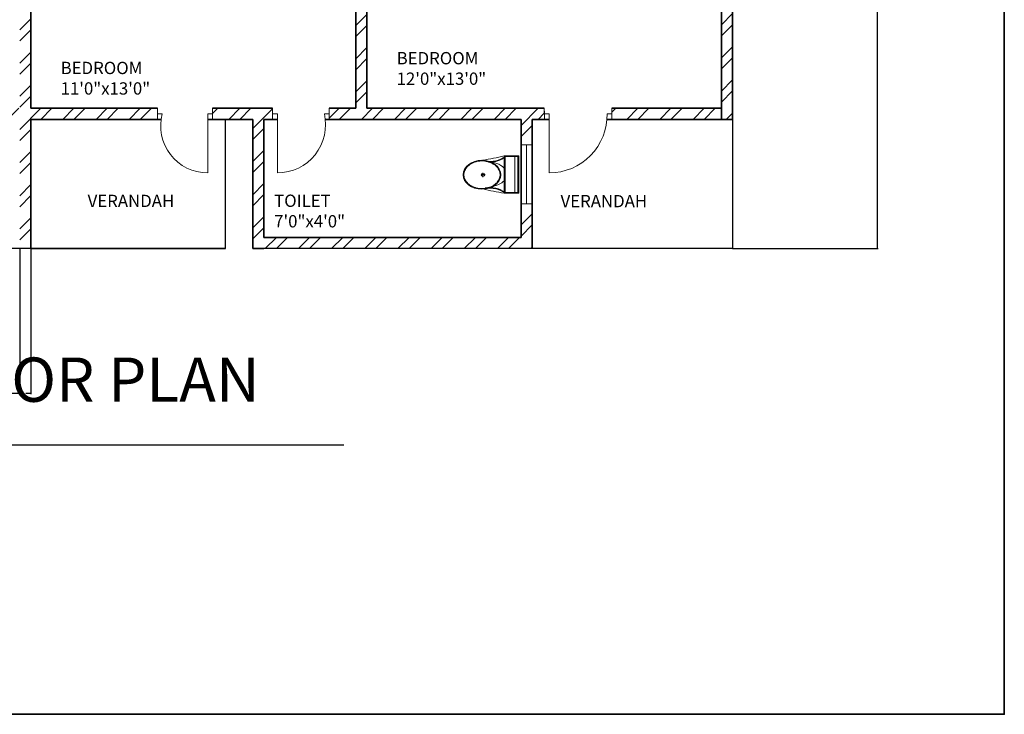
# Model space of a CAD drawing. Units: inches. Extents: x 1962 to 2771, y 1245 to 2660.
# Tile 8 of 114: x 2371 to 2771, y 1245 to 1527. Entities that reach past the tile are written whole.
import ezdxf

# ---------------------------------------------------------------- set-up
doc = ezdxf.new("R2010")
doc.units = ezdxf.units.IN
for name, color, linetype, lineweight in [('A-ANNO-DIMS', 2, 'Continuous', 18), ('A-ANNO-TEXT', 7, 'Continuous', 25), ('A-ANNO-TTLB', 7, 'Continuous', 35), ('A-AREA-IDEN', 7, 'Continuous', 18), ('A-DOOR', 3, 'Continuous', 18), ('A-FLOR-BALC', 7, 'Continuous', 25), ('A-FLOR-FIXT', 8, 'Continuous', 18), ('A-GLAZ', 4, 'Continuous', 18), ('A-WALL', 7, 'Continuous', 35), ('A-WALL-PATT', 252, 'Continuous', 13)]:
    doc.layers.add(name, color=color, linetype=linetype, lineweight=lineweight)
doc.styles.get("Standard").update_dxf_attribs({"font": 'arial.ttf'})
doc.dimstyles.get("Standard").update_dxf_attribs({"dimtxt": 0.18, "dimasz": 0.18, "dimexe": 0.18, "dimexo": 0.0625, "dimgap": 0.09, "dimtad": 0, "dimtih": 1, "dimtoh": 1, "dimdec": 4, "dimzin": 0, "dimdsep": 46, "dimtxsty": 'Standard', "dimcen": 0.09, "dimadec": 0, "dimazin": 0, "dimtfac": 1, "dimtdec": 4, "dimtofl": 0, "dimtmove": 0, "dimatfit": 3, "dimfxl": 1, "dimtolj": 1, "dimtzin": 0, "dimarcsym": 0})

# ---------------------------------------------------------------- blocks, each defined once
blk = doc.blocks.new('A$C31115884')
for p, q in [((283, 498), (223, 498)), ((258, 466), (258, 523)), ((0, 200), (0, 0)), ((520, 200), (0, 200)), ((10, 190), (10, 10)), ((510, 190), (10, 190)), ((510, 10), (510, 190)), ((520, 0), (520, 200)), ((510, 54), (0, 54)), ((10, 10), (510, 10)), ((0, 0), (520, 0))]:
    blk.add_line(p, q)
blk.add_circle((256, 496), 23.6)
for centre, radius, start, end in [((2778, -205), 2807, 165.4549, 171.7133), ((-295, 403), 365, 324.2091, 9.3499), ((-295, 403), 375, 324.2091, 9.3499), ((139, 406), 293, 315.8436, 2.6563), ((806, 403), 365, 170.6501, 215.7909), ((3237, 905), 2807, 188.2867, 194.5451), ((384, 406), 293, 190.2774, 224.1564), ((806, 403), 375, 179.2036, 215.7909)]:
    blk.add_arc(centre, radius, start, end)
blk.add_ellipse((256, 510), major_axis=(0, -261), ratio=0.772727)
blk.add_open_spline([(256, 259), (263, 259), (270, 260), (288, 262), (299, 265), (320, 273), (330, 278), (350, 291), (360, 299), (378, 316), (386, 326), (402, 347), (409, 358), (421, 383), (427, 395), (436, 422), (440, 436), (445, 465), (447, 480), (448, 509), (448, 524), (445, 553), (443, 568), (436, 596), (432, 610), (422, 636), (416, 649), (402, 672), (395, 683), (379, 703), (370, 712), (351, 728), (341, 735), (321, 746), (310, 751), (289, 757), (278, 759), (256, 761), (245, 761), (223, 757), (212, 754), (191, 746), (181, 741), (161, 728), (151, 720), (133, 703), (125, 693), (110, 672), (103, 660), (90, 636), (85, 623), (76, 596), (72, 582), (67, 553), (66, 538), (64, 509), (65, 494), (68, 465), (70, 450), (77, 422), (81, 408), (91, 382), (97, 370), (111, 346), (118, 335), (135, 316), (144, 307), (162, 291), (172, 284), (193, 273), (203, 269), (225, 262), (236, 260), (250, 259), (253, 259), (256, 259)], degree=3, knots=[0, 0, 0, 0, 0.110105, 0.110105, 0.285049, 0.285049, 0.459994, 0.459994, 0.634938, 0.634938, 0.809882, 0.809882, 0.984827, 0.984827, 1.159771, 1.159771, 1.334715, 1.334715, 1.50966, 1.50966, 1.684604, 1.684604, 1.859549, 1.859549, 2.034493, 2.034493, 2.209437, 2.209437, 2.384382, 2.384382, 2.559326, 2.559326, 2.73427, 2.73427, 2.909215, 2.909215, 3.084159, 3.084159, 3.259103, 3.259103, 3.434048, 3.434048, 3.608992, 3.608992, 3.783936, 3.783936, 3.958881, 3.958881, 4.133825, 4.133825, 4.30877, 4.30877, 4.483714, 4.483714, 4.658658, 4.658658, 4.833603, 4.833603, 5.008547, 5.008547, 5.183491, 5.183491, 5.358436, 5.358436, 5.53338, 5.53338, 5.708324, 5.708324, 5.883269, 5.883269, 6.058213, 6.058213, 6.233158, 6.233158, 6.283185, 6.283185, 6.283185, 6.283185])
blk = doc.blocks.new('WIN-24IN-A')
for p, q in [((0, 24), (4.5, 24)), ((4.5, 24), (2.25, 24)), ((2.25, 24), (2.25, 0)), ((2.25, 0), (0, 0)), ((0, 0), (4.5, 0))]:
    blk.add_line(p, q)
blk = doc.blocks.new('*D42')
at = {"layer": 'A-ANNO-DIMS', "color": 0, "lineweight": -2, "transparency": 16777216}
for p, q in [((2660.87, 2524.34), (2719.94, 2524.34)), ((2719.76, 2524.16), (2719.76, 1979.28)), ((2719.76, 1434.02), (2719.76, 1978.91)), ((2660.87, 1433.84), (2719.94, 1433.84))]:
    blk.add_line(p, q, dxfattribs=at)
at = {"layer": 'A-ANNO-DIMS', "color": 0, "transparency": 16777216}
for points in [[(2719.73, 2524.16), (2719.79, 2524.16), (2719.76, 2524.34)], [(2719.73, 1434.02), (2719.79, 1434.02), (2719.76, 1433.84)]]:
    blk.add_solid(points, dxfattribs=at)
at = {"layer": 'Defpoints', "color": 0, "transparency": 16777216}
for p in [(2660.81, 2524.34), (2719.76, 2524.34), (2660.81, 1433.84)]:
    blk.add_point(p, dxfattribs=at)
at = {"layer": 'A-ANNO-DIMS', "color": 0, "transparency": 16777216, "insert": (2719.76, 1979.09), "char_height": 0.18, "attachment_point": 5}
blk.add_mtext('\\A1;1090.5', dxfattribs=at)
blk = doc.blocks.new('*D46')
at = {"layer": 'A-ANNO-DIMS', "color": 0, "lineweight": -2, "transparency": 16777216}
for p, q in [((2086.31, 1433.78), (2086.31, 1374.71)), ((2371.31, 1433.78), (2371.31, 1374.71)), ((2086.49, 1374.89), (2228.52, 1374.89)), ((2371.13, 1374.89), (2229.1, 1374.89))]:
    blk.add_line(p, q, dxfattribs=at)
at = {"layer": 'A-ANNO-DIMS', "color": 0, "transparency": 16777216}
for points in [[(2086.49, 1374.92), (2086.49, 1374.86), (2086.31, 1374.89)], [(2371.13, 1374.92), (2371.13, 1374.86), (2371.31, 1374.89)]]:
    blk.add_solid(points, dxfattribs=at)
at = {"layer": 'Defpoints', "color": 0, "transparency": 16777216}
for p in [(2086.31, 1433.84), (2371.31, 1433.84), (2086.31, 1374.89)]:
    blk.add_point(p, dxfattribs=at)
at = {"layer": 'A-ANNO-DIMS', "color": 0, "transparency": 16777216, "insert": (2228.81, 1374.89), "char_height": 0.18, "attachment_point": 5}
blk.add_mtext('\\A1;285', dxfattribs=at)
blk = doc.blocks.new('*D48')
at = {"layer": 'A-ANNO-DIMS', "color": 0, "lineweight": -2, "transparency": 16777216}
for p, q in [((2371.31, 1433.78), (2371.31, 1374.71)), ((2375.81, 1433.78), (2375.81, 1374.71)), ((2371.49, 1374.89), (2373.3, 1374.89)), ((2375.63, 1374.89), (2373.82, 1374.89))]:
    blk.add_line(p, q, dxfattribs=at)
at = {"layer": 'A-ANNO-DIMS', "color": 0, "transparency": 16777216}
for points in [[(2371.49, 1374.92), (2371.49, 1374.86), (2371.31, 1374.89)], [(2375.63, 1374.92), (2375.63, 1374.86), (2375.81, 1374.89)]]:
    blk.add_solid(points, dxfattribs=at)
at = {"layer": 'Defpoints', "color": 0, "transparency": 16777216}
for p in [(2371.31, 1433.84), (2375.81, 1433.84), (2371.31, 1374.89)]:
    blk.add_point(p, dxfattribs=at)
at = {"layer": 'A-ANNO-DIMS', "color": 0, "transparency": 16777216, "insert": (2373.56, 1374.89), "char_height": 0.18, "attachment_point": 5}
blk.add_mtext('\\A1;4.5', dxfattribs=at)

msp = doc.modelspace()

# ---------------------------------------------------------------- hatches: boundary and pattern name
at = {"layer": 'A-WALL-PATT'}
h = msp.add_hatch(dxfattribs=at)
h.set_pattern_fill('ANSI32', color=256)
h.paths.add_polyline_path([(2090.8074, 2467.3437), (2141.6481, 2467.3437), (2141.6481, 2469.5937), (2141.6481, 2471.8437), (2086.3074, 2471.8437), (2086.3074, 2422.5333), (2090.8074, 2422.5333)])
h.paths.add_polyline_path([(2282.7664, 2471.8437), (2204.8982, 2471.8437), (2204.8982, 2467.3437), (2234.8074, 2467.3437), (2234.8074, 2311.3437), (2228.7492, 2311.3437), (2228.7492, 2306.8437), (2234.8074, 2306.8437), (2331.9227, 2306.8437), (2331.9227, 2309.0937), (2331.9227, 2311.3437), (2239.3074, 2311.3437), (2239.3074, 2467.3437), (2282.7664, 2467.3437), (2282.7664, 2469.5937)])
h.paths.add_polyline_path([(2471.4531, 2519.8437), (2552.011, 2519.8437), (2564.3996, 2519.8437), (2564.3996, 2511.1389), (2568.8996, 2511.1389), (2568.8996, 2524.3437), (2466.9531, 2524.3437), (2466.9531, 2471.8437), (2450.0749, 2471.8437), (2446.4672, 2471.8437), (2446.4672, 2467.3437), (2450.0749, 2467.3437), (2475.9988, 2467.3437), (2475.9988, 2469.5937), (2475.9988, 2471.8437), (2471.4531, 2471.8437)])
h.paths.add_polyline_path([(2575.2231, 2469.5937), (2575.2231, 2471.8437), (2568.8996, 2471.8437), (2568.8996, 2487.1389), (2564.3996, 2487.1389), (2564.3996, 2471.8437), (2556.511, 2471.8437), (2499.2904, 2471.8437), (2499.2904, 2467.3437), (2507.8074, 2467.3437), (2507.8074, 2311.3437), (2414.863, 2311.3437), (2414.863, 2306.8437), (2512.3074, 2306.8437), (2517.0114, 2306.8437), (2517.0114, 2309.0937), (2517.0114, 2311.3437), (2512.3074, 2311.3437), (2512.3074, 2467.3437), (2575.2231, 2467.3437)])
h.paths.add_polyline_path([(2660.8074, 2471.8437), (2600.9602, 2471.8437), (2600.9602, 2467.3437), (2656.3074, 2467.3437), (2656.3074, 2432.5704), (2660.8074, 2432.5704)])
h.paths.add_polyline_path([(2660.8074, 2372.5704), (2656.3074, 2372.5704), (2656.3074, 2311.3437), (2600.276, 2311.3437), (2600.276, 2309.0937), (2600.276, 2306.8437), (2656.3074, 2306.8437), (2656.3074, 2296.2593), (2660.8074, 2296.2593)])
h.paths.add_polyline_path([(2572.3074, 2306.8437), (2577.1385, 2306.8437), (2577.1385, 2311.3437), (2551.082, 2311.3437), (2551.082, 2306.8437), (2567.8074, 2306.8437), (2567.8074, 2258.8437), (2540.0574, 2258.8437), (2540.0574, 2256.5937), (2540.0574, 2254.3437), (2567.8074, 2254.3437), (2656.3074, 2254.3437), (2656.3074, 2236.9085), (2660.8074, 2236.9085), (2660.8074, 2272.2593), (2656.3074, 2272.2593), (2656.3074, 2258.8437), (2572.3074, 2258.8437)])
h.paths.add_polyline_path([(2512.3074, 2254.3437), (2518.8716, 2254.3437), (2518.8716, 2256.5937), (2518.8716, 2258.8437), (2507.8074, 2258.8437), (2507.8074, 2177.8437), (2567.8074, 2177.8437), (2567.8074, 2172.9628), (2572.3074, 2172.9628), (2572.3074, 2177.8437), (2656.3074, 2177.8437), (2656.3074, 2166.4846), (2660.8074, 2166.4846), (2660.8074, 2200.9085), (2656.3074, 2200.9085), (2656.3074, 2182.3437), (2512.3074, 2182.3437)])
h.paths.add_polyline_path([(2656.3074, 2129.8437), (2572.3074, 2129.8437), (2572.3074, 2150.3044), (2570.0574, 2150.3044), (2567.8074, 2150.3044), (2567.8074, 2129.8437), (2507.8074, 2129.8437), (2507.8074, 2116.3027), (2510.0574, 2116.3027), (2512.3074, 2116.3027), (2512.3074, 2125.3437), (2567.8074, 2125.3437), (2572.3074, 2125.3437), (2656.3074, 2125.3437)])
h.paths.add_polyline_path([(2090.8074, 2362.5333), (2086.3074, 2362.5333), (2086.3074, 2298.6242), (2090.8074, 2298.6242), (2090.8074, 2306.8437), (2174.8074, 2306.8437), (2174.8074, 2286.4178), (2179.3074, 2286.4178), (2179.3074, 2306.8437), (2192.8641, 2306.8437), (2192.8641, 2309.0937), (2192.8641, 2311.3437), (2090.8074, 2311.3437)])
h.paths.add_polyline_path([(2209.156, 2258.8437), (2179.3074, 2258.8437), (2179.3074, 2263.2236), (2177.0574, 2263.2236), (2174.8074, 2263.2236), (2174.8074, 2258.8437), (2090.8074, 2258.8437), (2090.8074, 2274.6242), (2086.3074, 2274.6242), (2086.3074, 2238.2967), (2088.5574, 2238.2967), (2090.8074, 2238.2967), (2090.8074, 2254.3437), (2209.156, 2254.3437)])
h.paths.add_polyline_path([(2090.8074, 2177.8437), (2234.8074, 2177.8437), (2234.8074, 2173.1428), (2239.3074, 2173.1428), (2239.3074, 2258.8437), (2230.8442, 2258.8437), (2230.8442, 2256.5937), (2230.8442, 2254.3437), (2234.8074, 2254.3437), (2234.8074, 2182.3437), (2090.8074, 2182.3437), (2090.8074, 2202.2967), (2086.3074, 2202.2967), (2086.3074, 2140.0389), (2090.8074, 2140.0389)])
h.paths.add_polyline_path([(2090.8074, 2080.0389), (2086.3074, 2080.0389), (2086.3074, 2033.8437), (2090.8074, 2033.8437)], flags=17)
h.paths.add_polyline_path([(2244.9405, 2033.8437), (2239.3074, 2033.8437), (2239.3074, 2142.0665), (2237.2592, 2142.0665), (2234.8074, 2142.0665), (2234.8074, 2033.8437), (2090.8074, 2033.8437), (2076.5204, 2033.8437), (2072.0204, 2033.8437), (2072.0204, 2000.4493), (2076.5204, 2000.4493), (2076.5204, 2029.3437), (2090.8074, 2029.3437), (2244.9405, 2029.3437), (2244.9405, 2031.5937)])
h.paths.add_polyline_path([(2234.8074, 1933.3437), (2076.5204, 1933.3437), (2076.5204, 1952.4493), (2074.2704, 1952.4493), (2072.0204, 1952.4493), (2072.0204, 1933.3437), (2072.0204, 1928.8437), (2234.8074, 1928.8437)])
h.paths.add_polyline_path([(2090.8074, 1928.8437), (2086.3074, 1928.8437), (2086.3074, 1906.5013), (2090.8074, 1906.5013)])
h.paths.add_polyline_path([(2090.8074, 1846.5013), (2086.3074, 1846.5013), (2086.3074, 1769.9917), (2088.5574, 1769.9917), (2090.8074, 1769.9917), (2090.8074, 1780.3437), (2234.8074, 1780.3437), (2234.8074, 1708.3437), (2230.3764, 1708.3437), (2230.3764, 1703.8437), (2239.3074, 1703.8437), (2239.3074, 1792.6669), (2237.0574, 1792.6669), (2234.8074, 1792.6669), (2234.8074, 1784.8437), (2090.8074, 1784.8437)])
h.paths.add_polyline_path([(2239.3074, 1928.8437), (2244.9405, 1928.8437), (2244.9405, 1931.0937), (2244.9405, 1933.3437), (2234.8074, 1933.3437), (2234.8074, 1928.8437), (2234.8074, 1825.5949), (2239.3074, 1825.5949)])
h.paths.add_polyline_path([(2148.0425, 1649.0937), (2148.0425, 1651.3437), (2090.8074, 1651.3437), (2090.8074, 1646.8437), (2148.0425, 1646.8437)], flags=0)
h.paths.add_polyline_path([(2207.5601, 1708.3437), (2090.8074, 1708.3437), (2090.8074, 1703.8437), (2174.8074, 1703.8437), (2174.8074, 1651.3437), (2170.4457, 1651.3437), (2170.4457, 1646.8437), (2195.9924, 1646.8437), (2195.9924, 1649.0937), (2195.9924, 1651.3437), (2179.3074, 1651.3437), (2179.3074, 1703.8437), (2207.5601, 1703.8437), (2207.5601, 1706.0937)])
h.paths.add_polyline_path([(2090.8074, 1733.9917), (2086.3074, 1733.9917), (2086.3074, 1696.1032), (2088.5574, 1696.1032), (2090.8074, 1696.1032)])
h.paths.add_polyline_path([(2090.8074, 1672.1032), (2086.3074, 1672.1032), (2086.3074, 1600.3335), (2090.8074, 1600.3335)])
h.paths.add_polyline_path([(2090.8074, 1540.3335), (2086.3074, 1540.3335), (2086.3074, 1486.3437), (2139.6766, 1486.3437), (2139.6766, 1490.8437), (2090.8074, 1490.8437)])
h.paths.add_polyline_path([(2302.3876, 1490.8437), (2239.3074, 1490.8437), (2239.3074, 1646.8437), (2335.9994, 1646.8437), (2335.9994, 1651.3437), (2229.884, 1651.3437), (2229.884, 1646.8437), (2234.8074, 1646.8437), (2234.8074, 1490.8437), (2202.7103, 1490.8437), (2202.7103, 1488.5937), (2202.7103, 1486.3437), (2275.0699, 1486.3437), (2275.0699, 1475.772), (2279.5699, 1475.772), (2279.5699, 1486.3437), (2302.3876, 1486.3437)])
h.paths.add_polyline_path([(2279.5699, 1451.772), (2275.0699, 1451.772), (2275.0699, 1438.3437), (2174.8074, 1438.3437), (2174.8074, 1486.3437), (2179.7922, 1486.3437), (2179.7922, 1490.8437), (2163.3585, 1490.8437), (2163.3585, 1488.5937), (2163.3585, 1486.3437), (2170.3074, 1486.3437), (2170.3074, 1433.8437), (2279.5699, 1433.8437)])
h.paths.add_polyline_path([(2427.2363, 1490.8437), (2375.8074, 1490.8437), (2375.8074, 1646.8437), (2381.6401, 1646.8437), (2381.6401, 1651.3437), (2365.887, 1651.3437), (2365.887, 1649.0937), (2365.887, 1646.8437), (2371.3074, 1646.8437), (2371.3074, 1490.8437), (2327.5627, 1490.8437), (2327.5627, 1488.5937), (2327.5627, 1486.3437), (2371.3074, 1486.3437), (2371.3074, 1433.8437), (2375.8074, 1433.8437), (2375.8074, 1486.3437), (2427.2363, 1486.3437)])
h.paths.add_polyline_path([(2512.3074, 1646.8437), (2519.4351, 1646.8437), (2519.4351, 1649.0937), (2519.4351, 1651.3437), (2507.8074, 1651.3437), (2416.0063, 1651.3437), (2416.0063, 1649.0937), (2416.0063, 1646.8437), (2507.8074, 1646.8437), (2507.8074, 1490.8437), (2497.0532, 1490.8437), (2497.0532, 1488.5937), (2497.0532, 1486.3437), (2574.9344, 1486.3437), (2574.9344, 1476.0181), (2579.4344, 1476.0181), (2579.4344, 1486.3437), (2584.4872, 1486.3437), (2584.3074, 1490.8437), (2512.3074, 1490.8437)])
h.paths.add_polyline_path([(2470.5091, 1486.3437), (2473.9767, 1486.3437), (2473.9767, 1490.8437), (2449.6605, 1490.8437), (2449.6605, 1488.5937), (2449.6605, 1486.3437), (2466.0091, 1486.3437), (2466.0091, 1433.8437), (2470.5091, 1433.8437), (2579.4344, 1433.8437), (2579.4344, 1452.0181), (2574.9344, 1452.0181), (2574.9344, 1438.3437), (2554.5091, 1438.3437), (2470.5091, 1438.3437)])
h.paths.add_polyline_path([(2656.3074, 1490.8437), (2611.86, 1490.8437), (2611.86, 1486.3437), (2656.3074, 1486.3437)])
h.paths.add_polyline_path([(2660.8074, 1532.7007), (2658.5574, 1532.7007), (2656.3074, 1532.7007), (2656.3074, 1486.3437), (2660.8074, 1486.3437)])
h.paths.add_polyline_path([(2660.8074, 1664.9663), (2656.3074, 1664.9663), (2656.3074, 1651.3437), (2602.2313, 1651.3437), (2602.2313, 1646.8437), (2656.3074, 1646.8437), (2656.3074, 1592.7007), (2660.8074, 1592.7007)])
h.paths.add_polyline_path([(2660.8074, 1724.5221), (2656.3074, 1724.5221), (2656.3074, 1703.8437), (2542.4725, 1703.8437), (2542.4725, 1699.3437), (2567.8074, 1699.3437), (2567.8074, 1651.3437), (2552.7766, 1651.3437), (2552.7766, 1649.0937), (2552.7766, 1646.8437), (2577.2878, 1646.8437), (2577.2878, 1649.0937), (2577.2878, 1651.3437), (2572.3074, 1651.3437), (2572.3074, 1699.3437), (2656.3074, 1699.3437), (2656.3074, 1688.9663), (2660.8074, 1688.9663)])
h.paths.add_polyline_path([(2660.8074, 1880.6524), (2656.3074, 1880.6524), (2656.3074, 1832.8437), (2512.3074, 1832.8437), (2512.3074, 1837.8959), (2507.8074, 1837.8959), (2507.8074, 1828.3437), (2567.8074, 1828.3437), (2567.8074, 1804.3437), (2572.3074, 1804.3437), (2572.3074, 1828.3437), (2656.3074, 1828.3437), (2656.3074, 1818.6778), (2660.8074, 1818.6778)])
h.paths.add_polyline_path([(2660.8074, 1794.6778), (2656.3074, 1794.6778), (2656.3074, 1780.3437), (2572.3074, 1780.3437), (2572.3074, 1783.0303), (2570.0574, 1783.0303), (2567.8074, 1783.0303), (2567.8074, 1780.3437), (2507.8074, 1780.3437), (2507.8074, 1699.3437), (2517.8858, 1699.3437), (2517.8858, 1701.5937), (2517.8858, 1703.8437), (2512.3074, 1703.8437), (2512.3074, 1775.8437), (2656.3074, 1775.8437), (2656.3074, 1760.5221), (2660.8074, 1760.5221)])
h.paths.add_polyline_path([(2660.8074, 1981.3437), (2660.8074, 2020.2808), (2658.5574, 2020.2808), (2656.3074, 2020.2808), (2656.3074, 1981.3437), (2512.3074, 1981.3437), (2512.3074, 2086.6996), (2507.8074, 2086.6996), (2507.8074, 1981.3437), (2375.8074, 1981.3437), (2375.8074, 1986.8505), (2373.5574, 1986.8505), (2371.3074, 1986.8505), (2371.3074, 1973.2607), (2375.8074, 1973.2607), (2375.8074, 1976.8437), (2507.8074, 1976.8437), (2507.8074, 1865.4281), (2510.0574, 1865.4281), (2512.3074, 1865.4281), (2512.3074, 1976.8437), (2660.8074, 1976.8437)])
h.paths.add_polyline_path([(2375.8074, 1940.297), (2373.5574, 1940.297), (2371.3074, 1940.297), (2371.3074, 1933.3437), (2278.4434, 1933.3437), (2278.4434, 1928.8437), (2371.3074, 1928.8437), (2371.3074, 1651.3437), (2375.8074, 1651.3437)])
h.paths.add_polyline_path([(2660.8074, 1976.8437), (2656.3074, 1976.8437), (2656.3074, 1940.6524), (2660.8074, 1940.6524)], flags=17)
h.paths.add_polyline_path([(2660.8074, 2142.4846), (2656.3074, 2142.4846), (2656.3074, 2080.2808), (2660.8074, 2080.2808)])
h.paths.add_polyline_path([(2381.4189, 2311.3437), (2375.8074, 2311.3437), (2375.8074, 2467.3437), (2424.7242, 2467.3437), (2424.7242, 2469.5937), (2424.7242, 2471.8437), (2375.8074, 2471.8437), (2375.8074, 2524.3437), (2371.3074, 2524.3437), (2371.3074, 2471.8437), (2307.2097, 2471.8437), (2307.2097, 2467.3437), (2371.3074, 2467.3437), (2371.3074, 2311.3437), (2366.8901, 2311.3437), (2366.8901, 2306.8437), (2371.3074, 2306.8437), (2371.3074, 2033.8437), (2279.6589, 2033.8437), (2279.6589, 2029.3437), (2371.3074, 2029.3437), (2371.3074, 2014.2598), (2375.8074, 2014.2598), (2375.8074, 2306.8437), (2381.4189, 2306.8437)])
h.paths.add_polyline_path([(2263.3074, 2524.3437), (2170.3074, 2524.3437), (2170.3074, 2519.8437), (2170.3074, 2471.8437), (2165.0312, 2471.8437), (2165.0312, 2467.3437), (2179.6721, 2467.3437), (2179.6721, 2469.5161), (2179.6721, 2471.8437), (2174.8074, 2471.8437), (2174.8074, 2519.8437), (2258.8074, 2519.8437), (2258.8074, 2511.6436), (2263.3074, 2511.6436)])
h.paths.add_polyline_path([(2245.0232, 1361.4123), (2492.9468, 1361.4123), (2492.9468, 1398.505), (2245.0232, 1398.505)], flags=9)
h.paths.add_polyline_path([(2388.1434, 2086.6936), (2425.0704, 2086.6936), (2425.0704, 2105.3509), (2388.1434, 2105.3509)], flags=9)
h.paths.add_polyline_path([(2404.922, 2242.6744), (2445.7337, 2242.6744), (2445.7337, 2261.3318), (2404.922, 2261.3318)], flags=9)
h.paths.add_polyline_path([(2269.4107, 2156.7935), (2306.3378, 2156.7935), (2306.3378, 2175.4508), (2269.4107, 2175.4508)], flags=9)
h.paths.add_polyline_path([(2269.3277, 2233.4343), (2306.2547, 2233.4343), (2306.2547, 2252.0917), (2269.3277, 2252.0917)], flags=9)
h.paths.add_polyline_path([(2431.6052, 2320.6922), (2470.4456, 2320.6922), (2470.4456, 2339.3495), (2431.6052, 2339.3495)], flags=25)
h.paths.add_polyline_path([(2249.6902, 2315.7608), (2288.5306, 2315.7608), (2288.5306, 2334.4182), (2249.6902, 2334.4182)], flags=25)
h.paths.add_polyline_path([(2096.9301, 2314.3181), (2135.7704, 2314.3181), (2135.7704, 2332.9755), (2096.9301, 2332.9755)], flags=25)
h.paths.add_polyline_path([(2134.3475, 2285.7089), (2161.4655, 2285.7089), (2161.4655, 2304.3662), (2134.3475, 2304.3662)], flags=9)
h.paths.add_polyline_path([(2126.5155, 2209.4076), (2159.9227, 2209.4076), (2159.9227, 2228.065), (2126.5155, 2228.065)], flags=25)
h.paths.add_polyline_path([(2110.5753, 2141.5299), (2149.4157, 2141.5299), (2149.4157, 2160.1872), (2110.5753, 2160.1872)], flags=25)
h.paths.add_polyline_path([(2249.8618, 1968.3317), (2286.3966, 1968.3317), (2286.3966, 1986.989), (2249.8618, 1986.989)], flags=9)
h.paths.add_polyline_path([(2395.9507, 1777.0051), (2436.7624, 1777.0051), (2436.7624, 1795.6625), (2395.9507, 1795.6625)], flags=9)
h.paths.add_polyline_path([(2398.5259, 1888.5651), (2435.0062, 1888.5651), (2435.0062, 1907.2224), (2398.5259, 1907.2224)], flags=25)
h.paths.add_polyline_path([(2259.3506, 1728.3559), (2296.2776, 1728.3559), (2296.2776, 1747.0132), (2259.3506, 1747.0132)], flags=9)
h.paths.add_polyline_path([(2271.3698, 1845.268), (2308.2968, 1845.268), (2308.2968, 1863.9253), (2271.3698, 1863.9253)], flags=9)
h.paths.add_polyline_path([(2120.9355, 1786.3027), (2159.7759, 1786.3027), (2159.7759, 1804.9601), (2120.9355, 1804.9601)], flags=25)
h.paths.add_polyline_path([(2121.3164, 1732.1043), (2154.7236, 1732.1043), (2154.7236, 1750.7616), (2121.3164, 1750.7616)], flags=25)
h.paths.add_polyline_path([(2118.3706, 1678.8997), (2147.5282, 1678.8997), (2147.5282, 1697.557), (2118.3706, 1697.557)], flags=25)
h.paths.add_polyline_path([(2385.9227, 1493.557), (2424.763, 1493.557), (2424.763, 1512.2143), (2385.9227, 1512.2143)], flags=25)
h.paths.add_polyline_path([(2248.7058, 1500.0256), (2287.5462, 1500.0256), (2287.5462, 1518.6829), (2248.7058, 1518.6829)], flags=25)
h.paths.add_polyline_path([(2104.1669, 1617.3771), (2143.0073, 1617.3771), (2143.0073, 1636.0344), (2104.1669, 1636.0344)], flags=9)
h.paths.add_polyline_path([(2096.0714, 1447.8824), (2137.3845, 1447.8824), (2137.3845, 1458.1859), (2096.0714, 1458.1859)], flags=9)
h.paths.add_polyline_path([(2180.6114, 1440.325), (2209.7689, 1440.325), (2209.7689, 1458.9823), (2180.6114, 1458.9823)], flags=25)
h.paths.add_polyline_path([(2316.1698, 1447.9637), (2357.4829, 1447.9637), (2357.4829, 1458.2673), (2316.1698, 1458.2673)], flags=9)
h.paths.add_polyline_path([(2397.6187, 1447.9637), (2438.9318, 1447.9637), (2438.9318, 1458.2673), (2397.6187, 1458.2673)], flags=9)
h.paths.add_polyline_path([(2473.0778, 1439.5953), (2502.2354, 1439.5953), (2502.2354, 1458.2527), (2473.0778, 1458.2527)], flags=25)
h.paths.add_polyline_path([(2589.7027, 1447.8819), (2631.0158, 1447.8819), (2631.0158, 1458.1855), (2589.7027, 1458.1855)], flags=9)
h.paths.add_polyline_path([(2522.4009, 1497.5285), (2561.2413, 1497.5285), (2561.2413, 1516.1859), (2522.4009, 1516.1859)], flags=25)
h.paths.add_polyline_path([(2579.6565, 1671.3482), (2608.8141, 1671.3482), (2608.8141, 1690.0056), (2579.6565, 1690.0056)], flags=25)
h.paths.add_polyline_path([(2544.7038, 1725.5064), (2578.1111, 1725.5064), (2578.1111, 1744.1637), (2544.7038, 1744.1637)], flags=25)
h.paths.add_polyline_path([(2578.1191, 1807.472), (2607.2766, 1807.472), (2607.2766, 1826.1293), (2578.1191, 1826.1293)], flags=25)
h.paths.add_polyline_path([(2595.0614, 1835.1839), (2633.9018, 1835.1839), (2633.9018, 1853.8413), (2595.0614, 1853.8413)], flags=25)
h.paths.add_polyline_path([(2567.0097, 2097.7035), (2605.8501, 2097.7035), (2605.8501, 2116.3609), (2567.0097, 2116.3609)], flags=9)
h.paths.add_polyline_path([(2586.644, 2134.6454), (2615.8015, 2134.6454), (2615.8015, 2153.3027), (2586.644, 2153.3027)], flags=9)
h.paths.add_polyline_path([(2544.6185, 2212.6783), (2578.0258, 2212.6783), (2578.0258, 2231.3356), (2544.6185, 2231.3356)], flags=25)
h.paths.add_polyline_path([(2577.0273, 2256.9023), (2606.1849, 2256.9023), (2606.1849, 2275.5597), (2577.0273, 2275.5597)], flags=24)
h.paths.add_polyline_path([(2605.2683, 2315.2821), (2644.1087, 2315.2821), (2644.1087, 2333.9395), (2605.2683, 2333.9395)], flags=25)
h.paths.add_polyline_path([(2583.1244, 2496.1815), (2624.4375, 2496.1815), (2624.4375, 2506.4851), (2583.1244, 2506.4851)], flags=9)
h.paths.add_polyline_path([(2474.761, 2497.0823), (2503.9185, 2497.0823), (2503.9185, 2515.7397), (2474.761, 2515.7397)], flags=25)
h.paths.add_polyline_path([(2387.5787, 2494.2563), (2428.902, 2494.2563), (2428.902, 2504.5598), (2387.5787, 2504.5598)], flags=9)
h.paths.add_polyline_path([(2300.1657, 2500.1564), (2341.4788, 2500.1564), (2341.4788, 2510.46), (2300.1657, 2510.46)], flags=25)
h.paths.add_polyline_path([(2176.8589, 2497.5843), (2206.0165, 2497.5843), (2206.0165, 2516.2416), (2176.8589, 2516.2416)], flags=25)
h.paths.add_polyline_path([(2097.4668, 2494.9762), (2138.7799, 2494.9762), (2138.7799, 2505.2798), (2097.4668, 2505.2798)], flags=9)

# ---------------------------------------------------------------- linework, layer by layer
at = {"layer": 'A-ANNO-TEXT'}
msp.add_line((2237.9561, 1354.1083), (2502.9067, 1354.1083), dxfattribs=at)
at = {"layer": 'A-ANNO-TTLB'}
msp.add_lwpolyline([(1961.7365, 2660.2579), (2771.213, 2660.2579), (2771.213, 1244.5817), (1961.7365, 1244.5817)], close=True, dxfattribs=at)
at = {"layer": 'A-DOOR'}
for p, q in [((2427.2363, 1486.3437), (2427.2363, 1490.8437)), ((2427.2363, 1490.8437), (2427.2363, 1488.5937)), ((2427.2363, 1488.5937), (2429.2363, 1488.5937)), ((2449.6605, 1488.5937), (2447.6605, 1488.5937)), ((2447.6605, 1488.5937), (2447.6605, 1464.5937)), ((2449.6605, 1486.3437), (2449.6605, 1490.8437)), ((2449.6605, 1490.8437), (2449.6605, 1488.5937)), ((2473.9767, 1486.3437), (2473.9767, 1490.8437)), ((2473.9767, 1490.8437), (2473.9767, 1488.5937)), ((2473.9767, 1488.5937), (2475.9767, 1488.5937)), ((2475.9767, 1488.5937), (2475.9767, 1464.5937)), ((2497.0532, 1488.5937), (2495.0532, 1488.5937)), ((2497.0532, 1486.3437), (2497.0532, 1490.8437)), ((2497.0532, 1490.8437), (2497.0532, 1488.5937)), ((2584.4872, 1486.3437), (2584.3074, 1490.8437)), ((2584.3074, 1490.8437), (2584.3973, 1488.5937)), ((2584.3973, 1488.5937), (2586.3973, 1488.5937)), ((2586.3973, 1488.5937), (2586.3973, 1464.5937)), ((2611.86, 1488.5937), (2609.86, 1488.5937)), ((2611.86, 1490.8437), (2611.86, 1486.3437)), ((2611.86, 1486.3437), (2611.86, 1488.5937))]:
    msp.add_line(p, q, dxfattribs=at)
for centre, radius, start, end in [((2447.6605, 1483.6656), 19.0719, 165.025087, 270), ((2475.9767, 1484.1752), 19.5815, 270, 13.040781), ((2586.3973, 1488.0624), 23.4687, 270, 1.297296)]:
    msp.add_arc(centre, radius, start, end, dxfattribs=at)
at = {"layer": 'A-FLOR-BALC'}
for p, q in [((2454.9439, 1433.8437), (2454.9439, 1486.3437)), ((2660.8074, 1486.3437), (2660.8074, 1433.8437)), ((2454.9439, 1433.8437), (2296.3835, 1433.8437)), ((2375.8074, 1433.8437), (2454.9439, 1433.8437)), ((2660.8074, 1433.8437), (2466.0091, 1433.8437))]:
    msp.add_line(p, q, dxfattribs=at)
at = {"layer": 'A-WALL'}
for p, q in [((2660.8074, 1976.8437), (2660.8074, 1486.3437)), ((2375.8074, 1646.8437), (2375.8074, 1490.8437)), ((2507.8074, 1646.8437), (2507.8074, 1490.8437)), ((2512.3074, 1646.8437), (2512.3074, 1490.8437)), ((2656.3074, 1646.8437), (2656.3074, 1486.3437)), ((2427.2363, 1490.8437), (2375.8074, 1490.8437)), ((2473.9767, 1490.8437), (2449.6605, 1490.8437)), ((2454.9439, 1490.8437), (2466.0091, 1490.8437)), ((2507.8074, 1490.8437), (2497.0532, 1490.8437)), ((2584.3074, 1490.8437), (2512.3074, 1490.8437)), ((2574.9344, 1490.8437), (2579.4344, 1490.8437)), ((2656.3074, 1490.8437), (2611.86, 1490.8437)), ((2375.8074, 1486.3437), (2375.8074, 1433.8437)), ((2428.7775, 1486.3437), (2375.8074, 1486.3437)), ((2466.0091, 1486.3437), (2447.6605, 1486.3437)), ((2466.0091, 1486.3437), (2466.0091, 1433.8437)), ((2470.5091, 1438.3437), (2470.5091, 1486.3437)), ((2475.9767, 1486.3437), (2470.5091, 1486.3437)), ((2574.9344, 1486.3437), (2495.4378, 1486.3437)), ((2574.9344, 1438.3437), (2574.9344, 1486.3437)), ((2579.4344, 1486.3437), (2579.4344, 1433.8437)), ((2586.3973, 1486.3437), (2579.4344, 1486.3437)), ((2656.3074, 1486.3437), (2609.803, 1486.3437)), ((2660.8074, 1486.3437), (2655.9821, 1486.3437)), ((2470.5091, 1438.3437), (2554.5091, 1438.3437)), ((2554.5091, 1438.3437), (2574.9344, 1438.3437)), ((2466.0091, 1433.8437), (2470.5091, 1433.8437))]:
    msp.add_line(p, q, dxfattribs=at)

# ---------------------------------------------------------------- block references
at = {"layer": 'A-FLOR-FIXT', "xscale": 0.0292470664339069, "yscale": 0.0292470664339069, "zscale": 0.0292470664339069, "rotation": 89.99999999999999}
msp.add_blockref('A$C31115884', (2573.9818, 1456.3331), dxfattribs=at)
at = {"layer": 'A-GLAZ'}
msp.add_blockref('WIN-24IN-A', (2574.9344, 1452.0181), dxfattribs=at)

# ---------------------------------------------------------------- texts
at = {"layer": 'A-ANNO-TEXT', "insert": (2251.5859, 1389.5603), "char_height": 18, "attachment_point": 1}
msp.add_mtext_dynamic_manual_height_columns('FIRST FLOOR PLAN', width=968.531758, gutter_width=12.5, heights=[0], dxfattribs=at)
at = {"layer": 'A-AREA-IDEN', "char_height": 5, "attachment_point": 1}
for s, width, insert in [('BEDROOM\\P12\'0"x13\'0"', 144.594142, (2524.4115, 1513.7012)), ('BEDROOM\\P11\'0"x13\'0"', 182.179647, (2387.9332, 1509.7297)), ('VERANDAH', 111.515445, (2398.8994, 1455.6939)), ('TOILET\\P7\'0"x4\'0"', 73.140905, (2474.6587, 1455.768)), ('VERANDAH', 141.792957, (2590.9834, 1455.6122))]:
    msp.add_mtext_dynamic_manual_height_columns(s, width=width, gutter_width=12.5, heights=[0], dxfattribs=dict(at, insert=insert))

# ---------------------------------------------------------------- dimensions: what is measured, and where the dimension line sits
at = {"layer": 'A-ANNO-DIMS'}
for base, p1, p2, angle, override, picture, middle in [((2719.7574, 2524.3437), (2660.8074, 1433.8437), (2660.8074, 2524.3437), 90, {"dimdec": 1, "dimlfac": 1, "dimrnd": 0, "dimzin": 0, "dimdsep": 46, "dimlunit": 2}, '*D42', (2719.7574, 1979.0937)), ((2086.3074, 1374.8937), (2371.3074, 1433.8437), (2086.3074, 1433.8437), 180, {"dimdec": 0, "dimlfac": 1, "dimrnd": 0, "dimzin": 0, "dimdsep": 46, "dimlunit": 2}, '*D46', (2228.8074, 1374.8937)), ((2371.3074, 1374.8937), (2375.8074, 1433.8437), (2371.3074, 1433.8437), 180, {"dimdec": 1, "dimlfac": 1, "dimrnd": 0, "dimzin": 0, "dimdsep": 46, "dimlunit": 2}, '*D48', (2373.5574, 1374.8937))]:
    dim = msp.add_linear_dim(base=base, p1=p1, p2=p2, angle=angle, dimstyle='Standard', override=override, dxfattribs=at)
    dim.commit()
    dim.dimension.update_dxf_attribs({"geometry": picture, "text_midpoint": middle})

doc.saveas('drawing.dxf')
